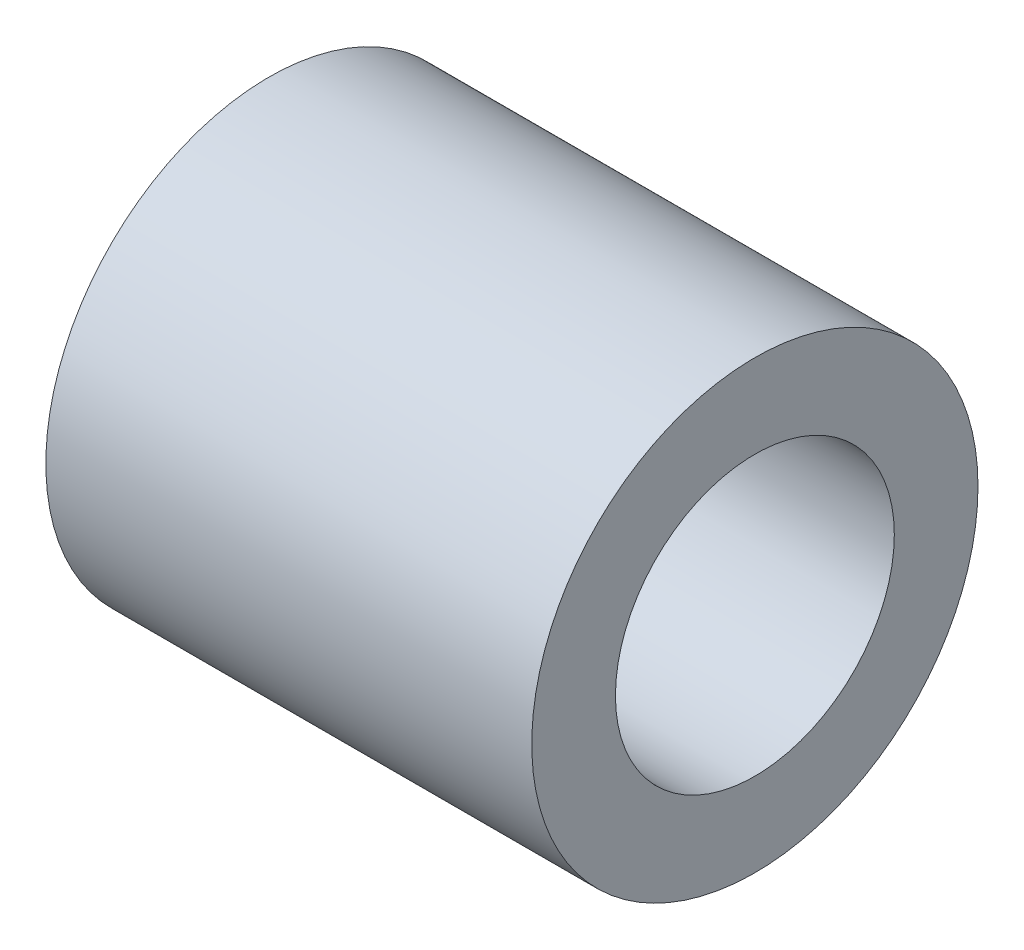
ISO-10303-21;
HEADER;
FILE_DESCRIPTION(('STEP AP214'),'2;1');
FILE_NAME('part.step','',(''),(''),'','','');
FILE_SCHEMA(('AUTOMOTIVE_DESIGN { 1 0 10303 214 1 1 1 1 }'));
ENDSEC;
DATA;
#1=APPLICATION_CONTEXT('core data for automotive mechanical design processes');
#2=APPLICATION_PROTOCOL_DEFINITION('international standard','automotive_design',2000,#1);
#3=PRODUCT_CONTEXT('',#1,'mechanical');
#4=PRODUCT('Part','Part','',(#3));
#5=PRODUCT_RELATED_PRODUCT_CATEGORY('part','',(#4));
#6=PRODUCT_DEFINITION_FORMATION('','',#4);
#7=PRODUCT_DEFINITION_CONTEXT('part definition',#1,'design');
#8=PRODUCT_DEFINITION('design','',#6,#7);
#9=PRODUCT_DEFINITION_SHAPE('','',#8);
#10=(LENGTH_UNIT() NAMED_UNIT(*) SI_UNIT(.MILLI.,.METRE.));
#11=(NAMED_UNIT(*) PLANE_ANGLE_UNIT() SI_UNIT($,.RADIAN.));
#12=(NAMED_UNIT(*) SI_UNIT($,.STERADIAN.) SOLID_ANGLE_UNIT());
#13=UNCERTAINTY_MEASURE_WITH_UNIT(LENGTH_MEASURE(1.E-05),#10,'distance_accuracy_value','');
#14=(GEOMETRIC_REPRESENTATION_CONTEXT(3) GLOBAL_UNCERTAINTY_ASSIGNED_CONTEXT((#13)) GLOBAL_UNIT_ASSIGNED_CONTEXT((#10,
#11,#12)) REPRESENTATION_CONTEXT('',''));
#15=CARTESIAN_POINT('',(0.,0.,0.));
#16=DIRECTION('',(0.,0.,1.));
#17=DIRECTION('',(1.,0.,0.));
#18=AXIS2_PLACEMENT_3D('',#15,#16,#17);
#19=CARTESIAN_POINT('',(9.,0.,0.));
#20=DIRECTION('',(-1.,0.,0.));
#21=DIRECTION('',(0.,0.,1.));
#22=AXIS2_PLACEMENT_3D('',#19,#20,#21);
#23=CYLINDRICAL_SURFACE('',#22,4.);
#24=CARTESIAN_POINT('',(9.,0.,0.));
#25=DIRECTION('',(1.,0.,0.));
#26=DIRECTION('',(0.,0.,-1.));
#27=AXIS2_PLACEMENT_3D('',#24,#25,#26);
#28=CIRCLE('',#27,4.);
#29=CARTESIAN_POINT('',(9.,0.,-4.));
#30=VERTEX_POINT('',#29);
#31=EDGE_CURVE('E10',#30,#30,#28,.T.);
#32=ORIENTED_EDGE('',*,*,#31,.F.);
#33=EDGE_LOOP('',(#32));
#34=FACE_BOUND('',#33,.T.);
#35=CARTESIAN_POINT('',(0.288675134594843,0.,0.));
#36=DIRECTION('',(1.,0.,0.));
#37=DIRECTION('',(0.,0.,-1.));
#38=AXIS2_PLACEMENT_3D('',#35,#36,#37);
#39=CIRCLE('',#38,4.);
#40=CARTESIAN_POINT('',(0.288675134594843,0.,-4.));
#41=VERTEX_POINT('',#40);
#42=EDGE_CURVE('E44',#41,#41,#39,.F.);
#43=ORIENTED_EDGE('',*,*,#42,.F.);
#44=EDGE_LOOP('',(#43));
#45=FACE_BOUND('',#44,.T.);
#46=ADVANCED_FACE('F39',(#34,#45),#23,.T.);
#47=CARTESIAN_POINT('',(9.,0.,0.));
#48=DIRECTION('',(1.,0.,0.));
#49=DIRECTION('',(0.,0.,-1.));
#50=AXIS2_PLACEMENT_3D('',#47,#48,#49);
#51=PLANE('',#50);
#52=CARTESIAN_POINT('',(9.,0.,0.));
#53=DIRECTION('',(1.,0.,0.));
#54=DIRECTION('',(0.,0.,-1.));
#55=AXIS2_PLACEMENT_3D('',#52,#53,#54);
#56=CIRCLE('',#55,2.5);
#57=CARTESIAN_POINT('',(9.,0.,-2.5));
#58=VERTEX_POINT('',#57);
#59=EDGE_CURVE('E57',#58,#58,#56,.T.);
#60=ORIENTED_EDGE('',*,*,#59,.F.);
#61=EDGE_LOOP('',(#60));
#62=FACE_BOUND('',#61,.T.);
#63=ORIENTED_EDGE('',*,*,#31,.T.);
#64=EDGE_LOOP('',(#63));
#65=FACE_BOUND('',#64,.T.);
#66=ADVANCED_FACE('F72',(#62,#65),#51,.T.);
#67=CARTESIAN_POINT('',(0.,0.,0.));
#68=DIRECTION('',(1.,0.,0.));
#69=DIRECTION('',(0.,0.,-1.));
#70=AXIS2_PLACEMENT_3D('',#67,#68,#69);
#71=CONICAL_SURFACE('',#70,3.5,1.04719755119655);
#72=CARTESIAN_POINT('',(0.,0.,0.));
#73=DIRECTION('',(-1.,0.,0.));
#74=DIRECTION('',(0.,0.,1.));
#75=AXIS2_PLACEMENT_3D('',#72,#73,#74);
#76=CIRCLE('',#75,3.5);
#77=CARTESIAN_POINT('',(0.,0.,3.5));
#78=VERTEX_POINT('',#77);
#79=EDGE_CURVE('E47',#78,#78,#76,.T.);
#80=ORIENTED_EDGE('',*,*,#79,.F.);
#81=EDGE_LOOP('',(#80));
#82=FACE_BOUND('',#81,.T.);
#83=ORIENTED_EDGE('',*,*,#42,.T.);
#84=EDGE_LOOP('',(#83));
#85=FACE_BOUND('',#84,.T.);
#86=ADVANCED_FACE('F71',(#82,#85),#71,.T.);
#87=CARTESIAN_POINT('',(0.,0.,0.));
#88=DIRECTION('',(1.,0.,0.));
#89=DIRECTION('',(0.,0.,-1.));
#90=AXIS2_PLACEMENT_3D('',#87,#88,#89);
#91=PLANE('',#90);
#92=ORIENTED_EDGE('',*,*,#79,.T.);
#93=EDGE_LOOP('',(#92));
#94=FACE_BOUND('',#93,.T.);
#95=ADVANCED_FACE('F69',(#94),#91,.F.);
#96=CARTESIAN_POINT('',(3.,0.,0.));
#97=DIRECTION('',(1.,0.,0.));
#98=DIRECTION('',(0.,0.,-1.));
#99=AXIS2_PLACEMENT_3D('',#96,#97,#98);
#100=CYLINDRICAL_SURFACE('',#99,2.5);
#101=CARTESIAN_POINT('',(3.,0.,0.));
#102=DIRECTION('',(1.,0.,0.));
#103=DIRECTION('',(0.,0.,-1.));
#104=AXIS2_PLACEMENT_3D('',#101,#102,#103);
#105=CIRCLE('',#104,2.5);
#106=CARTESIAN_POINT('',(3.,0.,-2.5));
#107=VERTEX_POINT('',#106);
#108=EDGE_CURVE('E52',#107,#107,#105,.T.);
#109=ORIENTED_EDGE('',*,*,#108,.F.);
#110=EDGE_LOOP('',(#109));
#111=FACE_BOUND('',#110,.T.);
#112=ORIENTED_EDGE('',*,*,#59,.T.);
#113=EDGE_LOOP('',(#112));
#114=FACE_BOUND('',#113,.T.);
#115=ADVANCED_FACE('F63',(#111,#114),#100,.F.);
#116=CARTESIAN_POINT('',(3.,0.,0.));
#117=DIRECTION('',(1.,0.,0.));
#118=DIRECTION('',(0.,0.,-1.));
#119=AXIS2_PLACEMENT_3D('',#116,#117,#118);
#120=PLANE('',#119);
#121=ORIENTED_EDGE('',*,*,#108,.T.);
#122=EDGE_LOOP('',(#121));
#123=FACE_BOUND('',#122,.T.);
#124=ADVANCED_FACE('F65',(#123),#120,.T.);
#125=CLOSED_SHELL('',(#46,#66,#86,#95,#115,#124));
#126=MANIFOLD_SOLID_BREP('B2',#125);
#127=ADVANCED_BREP_SHAPE_REPRESENTATION('',(#18,#126),#14);
#128=SHAPE_DEFINITION_REPRESENTATION(#9,#127);
ENDSEC;
END-ISO-10303-21;
